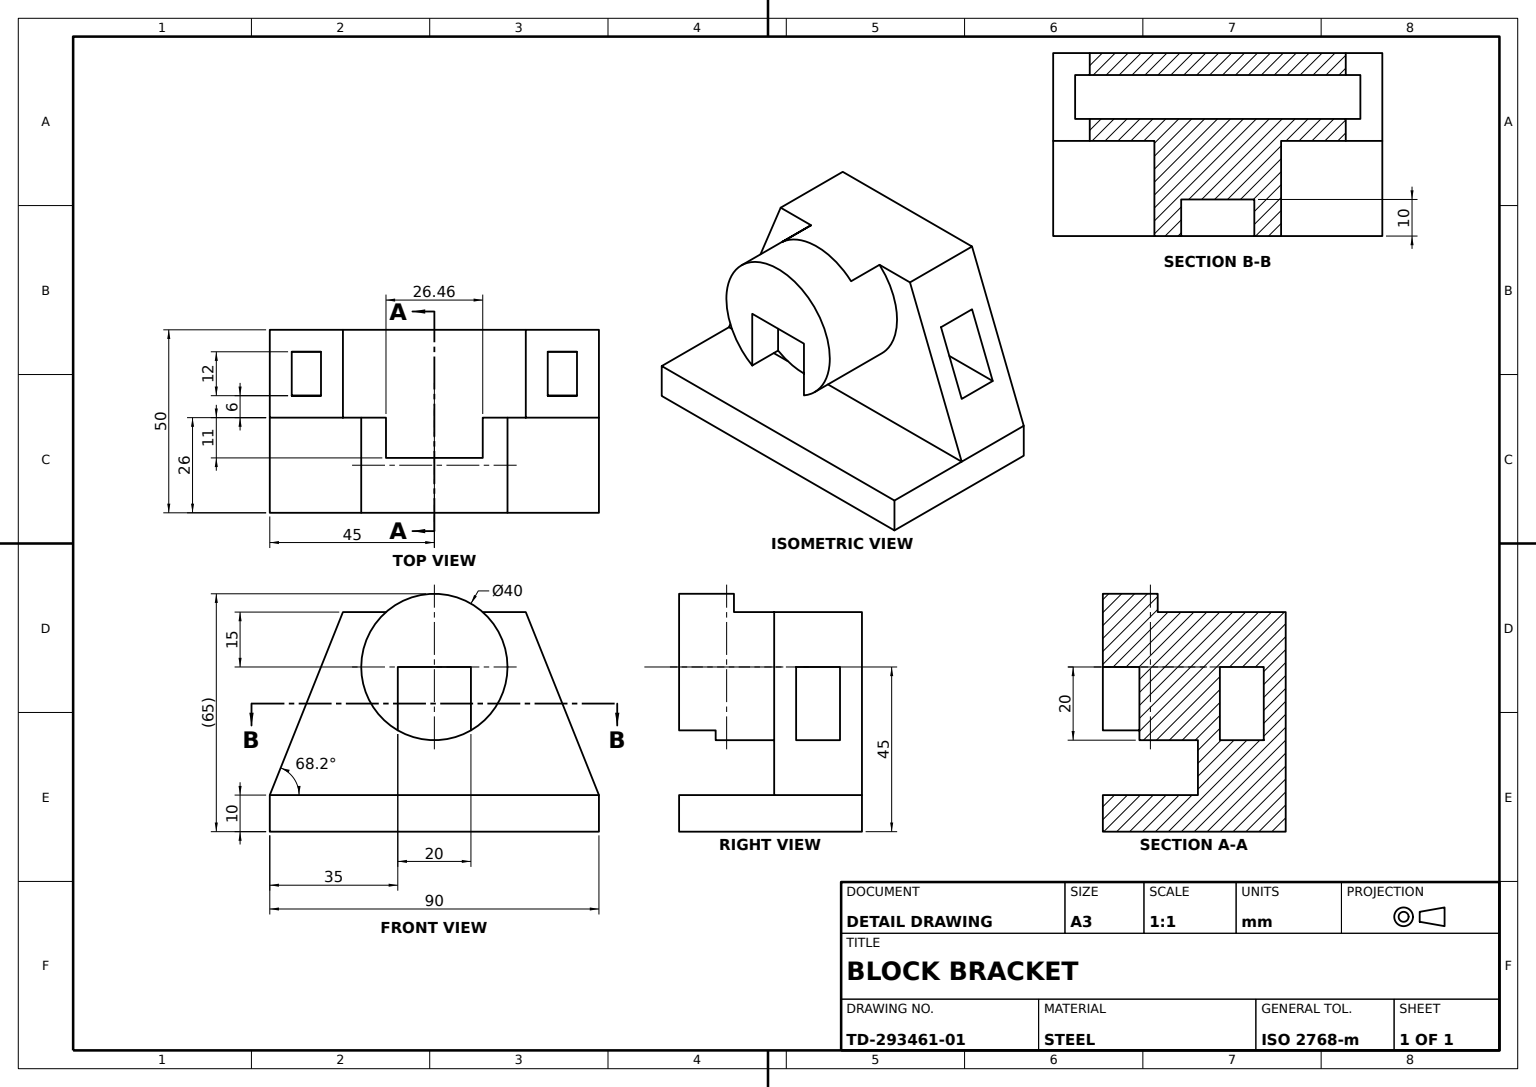
SolidWorks part; units mm, degrees
material "Plain Carbon Steel"
ref_plane "Front Plane" through (0, 0, 0) normal (0, 0, 1) x (1, 0, 0)
ref_plane "Top Plane" through (0, 0, 0) normal (0, 1, 0) x (1, 0, 0)
ref_plane "Right Plane" through (0, 0, 0) normal (1, 0, 0) x (0, 0, -1)
sketch "Base Plate Sketch" plane through (0, 0, 0) normal (0, 1, 0) x (1, 0, 0)
  line L1 (-25, -45) -> (25, -45)
  line L2 (-25, -45) -> (-25, 45)
  line L3 (-25, 45) -> (25, 45)
  line L4 (25, -45) -> (25, 45)
  line L5 (-25, -45) -> (25, 45) construction
  line L6 (-25, 45) -> (25, -45) construction
  point P0 (0, 0)
  dimension "D1" = 50
  dimension "D2" = 90
extrude "Base Plate 90x50x10" add sketch "Base Plate Sketch" along normal blind 10
sketch "Upright Web Sketch" plane through (-25, 0, 0) normal (-1, 0, 0) x (0, 0, 1)
  line L0 (0, 0) -> (0, 65.5698) construction
  line L1 (-25, 60) -> (25, 60)
  line L2 (25, 60) -> (45, 10)
  line L3 (-25, 60) -> (-45, 10)
  line L4 (-45, 10) -> (45, 10) construction
  line L5 (-45, 10) -> (45, 10)
  dimension "D1" = 50
  dimension "D2" = 25
  dimension "D3" = 50
extrude "Upright Web" add sketch "Upright Web Sketch" against normal blind 24
sketch "Web Window Sketch" plane through (0, 0, -45) normal (0, 0, -1) x (-1, 0, 0)
  line L0 (13, 60) -> (13, -7.2317) construction
  line L1 (1, 60) -> (25, 60) construction
  line L2 (1, 35) -> (25, 35) construction
  line L3 (1, 60) -> (1, 10) construction
  line L4 (25, 60) -> (25, 10) construction
  line L6 (7, 25) -> (19, 25)
  line L7 (7, 25) -> (7, 45)
  line L8 (7, 45) -> (19, 45)
  line L9 (19, 25) -> (19, 45)
  line L10 (7, 25) -> (19, 45) construction
  line L11 (7, 45) -> (19, 25) construction
  point P10 (13, 35)
  dimension "D1" = 20
  dimension "D2" = 6
  dimension "D3" = 15
extrude "Web Window Cut" cut sketch "Web Window Sketch" against normal blind 100 and the other way through all
sketch "Cylinder Boss Sketch" plane through (-1, 0, 0) normal (1, 0, 0) x (0, 0, -1)
  line L0 (0, 0) -> (0, 45) construction
  circle A0 centre (0, 45) radius 20
  dimension "D2" = 40
  dimension "D1" = 45
extrude "Cylinder Boss" add sketch "Cylinder Boss Sketch" along normal blind 26
sketch "Boss End Slot Sketch" plane through (25, 0, 0) normal (1, 0, 0) x (0, 0, -1)
  line L0 (0, 0) -> (0, 45) construction
  line L1 (-10, 45) -> (10, 45)
  line L2 (10, 45) -> (10, 27.6795)
  line L3 (-10, 45) -> (-10, 27.6795)
  arc A0 (-13.2288, 60) -> (13.2288, 60) centre (0, 45) ccw construction
  circle A1 centre (0, 45) radius 20 construction
  arc A2 (-10, 27.6795) -> (10, 27.6795) centre (0, 45) ccw
  dimension "D1" = 20
  dimension "D2" = 10
extrude "Boss End Slot 20x10" cut sketch "Boss End Slot Sketch" against normal blind 10 contours A2 L2 L1 L3
sketch "Top Notch Sketch" plane through (-1, 0, 0) normal (-1, 0, 0) x (0, 0, 1)
  line L1 (-13.2288, 60) -> (13.2288, 60)
  line L2 (-13.2288, 60) -> (13.2288, 60)
  arc A1 (13.2288, 60) -> (-13.2288, 60) centre (0, 45) ccw
  arc A2 (13.2288, 60) -> (-13.2288, 60) centre (0, 45) ccw
  dimension "D1" = 0
extrude "Top Notch Cut" cut sketch "Top Notch Sketch" against normal blind 11
